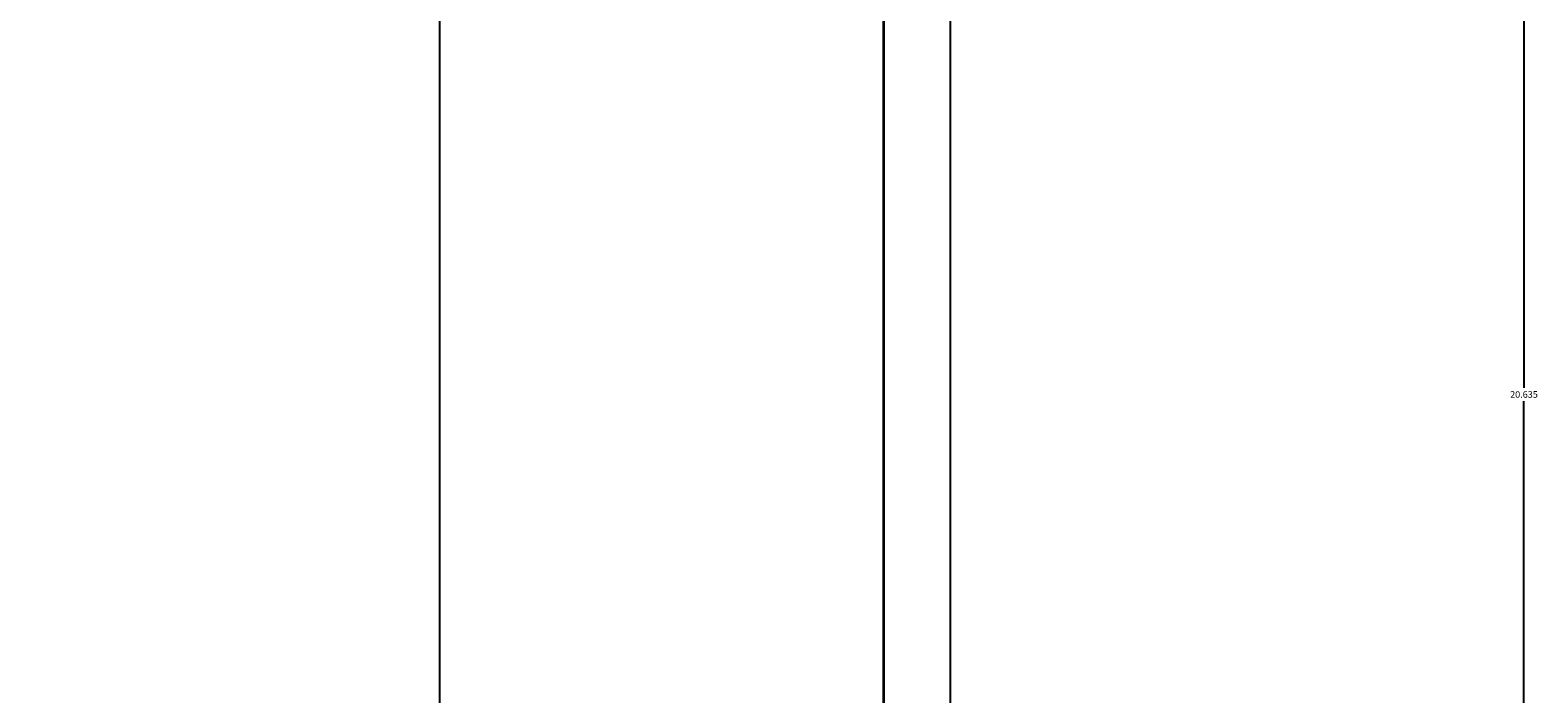
# Model space of a CAD drawing. Units: inches. Extents: x -6 to 289, y -8 to 323.
# Tile 97 of 107: x 248 to 289, y 229 to 247. Entities that reach past the tile are written whole.
import ezdxf

# ---------------------------------------------------------------- set-up
doc = ezdxf.new("R2010")
doc.units = ezdxf.units.IN
doc.header["$MEASUREMENT"] = 0
doc.layers.add('A-ANNO-DIMS', color=2, linetype='Continuous', lineweight=18)
doc.layers.add('A-ELEV', color=7, linetype='Continuous', lineweight=35)
doc.styles.get("Standard").update_dxf_attribs({"font": 'arial.ttf'})
doc.dimstyles.get("Standard").update_dxf_attribs({"dimtxt": 0.18, "dimasz": 0.18, "dimexe": 0.18, "dimexo": 0.0625, "dimgap": 0.09, "dimtad": 0, "dimtih": 1, "dimtoh": 1, "dimdec": 4, "dimzin": 0, "dimdsep": 46, "dimtxsty": 'Standard', "dimcen": 0.09, "dimadec": 0, "dimazin": 0, "dimtfac": 1, "dimtdec": 4, "dimtofl": 0, "dimtmove": 0, "dimatfit": 3, "dimfxl": 1, "dimtolj": 1, "dimtzin": 0, "dimarcsym": 0})

# ---------------------------------------------------------------- blocks, each defined once
blk = doc.blocks.new('*D15')
at = {"layer": 'A-ANNO-DIMS', "color": 0, "lineweight": -2, "transparency": 16777216}
for p, q in [((247.164, 162.411), (247.164, 322.969)), ((271.164, 7.351), (271.164, 322.969)), ((247.344, 322.789), (258.944, 322.789)), ((270.984, 322.789), (259.384, 322.789))]:
    blk.add_line(p, q, dxfattribs=at)
at = {"layer": 'A-ANNO-DIMS', "color": 0, "transparency": 16777216}
for points in [[(247.344, 322.819), (247.344, 322.759), (247.164, 322.789)], [(270.984, 322.819), (270.984, 322.759), (271.164, 322.789)]]:
    blk.add_solid(points, dxfattribs=at)
at = {"layer": 'Defpoints', "color": 0, "transparency": 16777216}
for p in [(271.164, 322.789), (247.164, 162.348), (271.164, 7.289)]:
    blk.add_point(p, dxfattribs=at)
at = {"layer": 'A-ANNO-DIMS', "color": 0, "transparency": 16777216, "insert": (259.164, 322.789), "char_height": 0.18, "attachment_point": 5}
blk.add_mtext('\\A1;24', dxfattribs=at)
blk = doc.blocks.new('*D26')
at = {"layer": 'A-ANNO-DIMS', "color": 0, "lineweight": -2, "transparency": 16777216}
for p, q in [((247.226, 247.289), (288.653, 247.289)), ((288.473, 247.109), (288.473, 237.153)), ((288.473, 226.834), (288.473, 236.789)), ((126.946, 226.654), (288.653, 226.654))]:
    blk.add_line(p, q, dxfattribs=at)
at = {"layer": 'A-ANNO-DIMS', "color": 0, "transparency": 16777216}
for points in [[(288.443, 247.109), (288.503, 247.109), (288.473, 247.289)], [(288.443, 226.834), (288.503, 226.834), (288.473, 226.654)]]:
    blk.add_solid(points, dxfattribs=at)
at = {"layer": 'Defpoints', "color": 0, "transparency": 16777216}
for p in [(247.164, 247.289), (288.473, 247.289), (126.883, 226.654)]:
    blk.add_point(p, dxfattribs=at)
at = {"layer": 'A-ANNO-DIMS', "color": 0, "transparency": 16777216, "insert": (288.473, 236.971), "char_height": 0.18, "attachment_point": 5}
blk.add_mtext('\\A1;20.635', dxfattribs=at)
blk = doc.blocks.new('*D82')
at = {"layer": 'A-ANNO-DIMS', "color": 0, "lineweight": -2, "transparency": 16777216}
for p, q in [((245.215, 66.286), (245.215, 322.969)), ((272.973, 66.286), (272.973, 322.969)), ((245.395, 322.789), (258.699, 322.789)), ((272.793, 322.789), (259.489, 322.789))]:
    blk.add_line(p, q, dxfattribs=at)
at = {"layer": 'A-ANNO-DIMS', "color": 0, "transparency": 16777216}
for points in [[(245.395, 322.819), (245.395, 322.759), (245.215, 322.789)], [(272.793, 322.819), (272.793, 322.759), (272.973, 322.789)]]:
    blk.add_solid(points, dxfattribs=at)
at = {"layer": 'Defpoints', "color": 0, "transparency": 16777216}
for p in [(272.973, 322.789), (245.215, 66.224), (272.973, 66.224)]:
    blk.add_point(p, dxfattribs=at)
at = {"layer": 'A-ANNO-DIMS', "color": 0, "transparency": 16777216, "insert": (259.094, 322.789), "char_height": 0.18, "attachment_point": 5}
blk.add_mtext('\\A1;27.76', dxfattribs=at)
blk = doc.blocks.new('*D100')
at = {"layer": 'A-ANNO-DIMS', "color": 0, "lineweight": -2, "transparency": 16777216}
for p, q in [((247.164, 162.411), (247.164, 322.969)), ((259.164, 139.351), (259.164, 322.969)), ((247.344, 322.789), (252.954, 322.789)), ((258.984, 322.789), (253.373, 322.789))]:
    blk.add_line(p, q, dxfattribs=at)
at = {"layer": 'A-ANNO-DIMS', "color": 0, "transparency": 16777216}
for points in [[(247.344, 322.819), (247.344, 322.759), (247.164, 322.789)], [(258.984, 322.819), (258.984, 322.759), (259.164, 322.789)]]:
    blk.add_solid(points, dxfattribs=at)
at = {"layer": 'Defpoints', "color": 0, "transparency": 16777216}
for p in [(259.164, 322.789), (247.164, 162.348), (259.164, 139.289)]:
    blk.add_point(p, dxfattribs=at)
at = {"layer": 'A-ANNO-DIMS', "color": 0, "transparency": 16777216, "insert": (253.164, 322.789), "char_height": 0.18, "attachment_point": 5}
blk.add_mtext('\\A1;12', dxfattribs=at)

msp = doc.modelspace()

# ---------------------------------------------------------------- linework, layer by layer
at = {"layer": 'A-ELEV'}
msp.add_line((271.1638, 68.4323), (271.1638, 259.2888), dxfattribs=at)

# ---------------------------------------------------------------- dimensions: what is measured, and where the dimension line sits
at = {"layer": 'A-ANNO-DIMS'}
for base, p1, p2, override, picture, middle in [((272.9733, 322.7888), (245.2146, 66.2238), (272.9733, 66.2238), {"dimdec": 2, "dimlfac": 1, "dimrnd": 0, "dimzin": 0, "dimdsep": 46, "dimlunit": 2}, '*D82', (259.0939, 322.7888)), ((271.1638, 322.7888), (247.1638, 162.3484), (271.1638, 7.2888), {"dimdec": 0, "dimlfac": 1, "dimrnd": 0, "dimzin": 0, "dimdsep": 46, "dimlunit": 2}, '*D15', (259.1638, 322.7888)), ((259.1638, 322.7888), (247.1638, 162.3484), (259.1638, 139.2888), {"dimdec": 0, "dimlfac": 1, "dimrnd": 0, "dimzin": 0, "dimdsep": 46, "dimlunit": 2}, '*D100', (253.1638, 322.7888))]:
    dim = msp.add_linear_dim(base=base, p1=p1, p2=p2, dimstyle='Standard', override=override, dxfattribs=at)
    dim.commit()
    dim.dimension.update_dxf_attribs({"geometry": picture, "text_midpoint": middle})
dim = msp.add_linear_dim(base=(288.4733, 247.2888), p1=(126.8835, 226.654), p2=(247.1638, 247.2888), angle=90, dimstyle='Standard', override={"dimdec": 3, "dimlfac": 1, "dimrnd": 0, "dimzin": 0, "dimdsep": 46, "dimlunit": 2}, dxfattribs=at)
dim.commit()
dim.dimension.update_dxf_attribs({"geometry": '*D26', "text_midpoint": (288.4733, 236.9714)})

doc.saveas('drawing.dxf')
